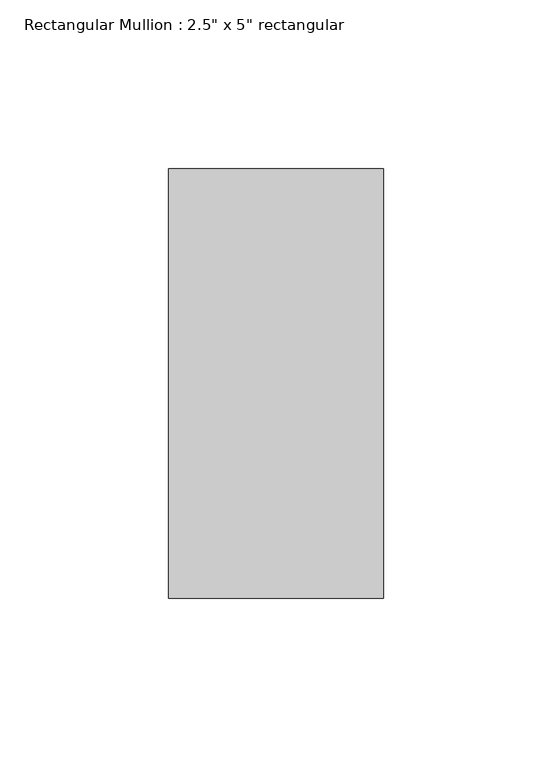
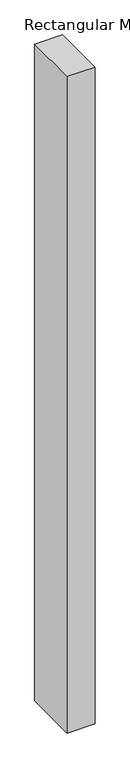
"""IFC4 building model written with IfcOpenShell, lengths in millimetres: member geometry."""

from ifc_helpers import new_model, si_unit, frame, origin, place, context, project, spatial, polyline, outline, extrude, source, transform, mapped, element, save


def member_dfbe775a(model_context):
    return source(origin(), model_context, "Body", "SweptSolid", [
        extrude(outline(polyline([(31.75, 63.5), (31.75, -63.5), (-31.75, -63.5), (-31.75, 63.5), (31.75, 63.5)])), frame((0.0, 0.0, -1574.2288132), z_axis=(0.0, 0.0, 1.0), x_axis=(1.0, 0.0, 0.0)), (0.0, 0.0, 1.0), 1574.2288132),
    ])


if __name__ == "__main__":
    model = new_model("IFC4")
    model_context = context("Model", 3, world=origin())
    ifc_project = project(units=[si_unit("LENGTHUNIT", "METRE", prefix="MILLI")], contexts=[model_context])
    site = spatial("IfcSite", under=ifc_project)
    building = spatial("IfcBuilding", under=site)
    placement = place(None, origin())
    member_shape = member_dfbe775a(model_context)
    element("IfcMember", 1, ObjectType="Rectangular Mullion : 2.5\" x 5\" rectangular", at=placement, inside=building, context=model_context, shape_type="MappedRepresentation", body=[
        mapped(member_shape, transform((0.0, 0.0, 0.0), x_axis=(1.0, 0.0, 0.0), y_axis=(0.0, 1.0, 0.0), z_axis=(0.0, 0.0, 1.0))),
    ])
    save(model, "model.ifc")

# Revit data of these elements
# Type "Rectangular Mullion : 2.5\" x 5\" rectangular"
#   built-in parameter 1007304 = 0.416667 (stored number, unit not read)
#   built-in parameter 1007301 = 0.104167 (stored number, unit not read)
#   built-in parameter 1007300 = 0.104167 (stored number, unit not read)
# Element 1 (IfcMember, "Rectangular Mullion : 2.5\" x 5\" rectangular")
#   Materials on its faces: "Aluminum"
# Materials
#   "Aluminum": class "Metal", colour RGB 247 247 247, transparency 0, Description = "Aluminum 6061", Cost = 0
